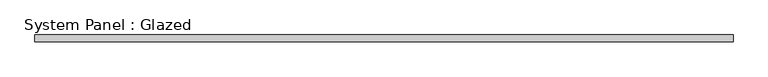
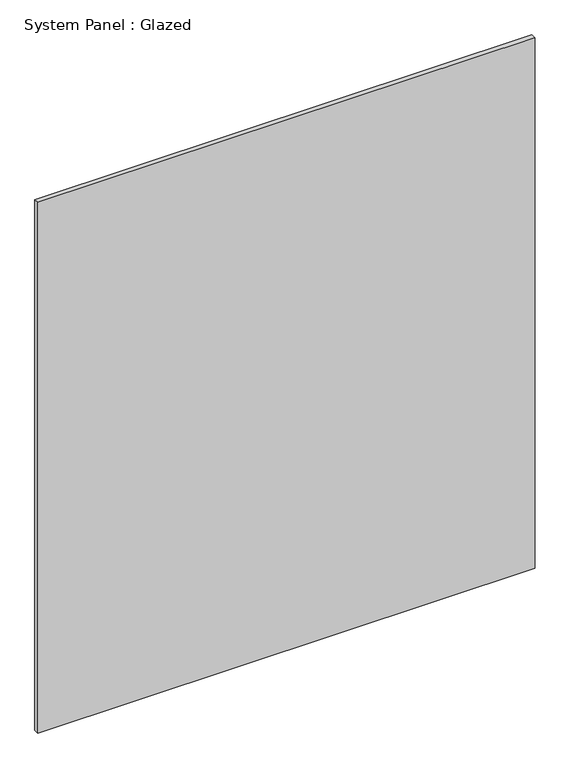
"""IFC4 building model written with IfcOpenShell, lengths in millimetres: plate geometry, System Panel : Glazed."""

from ifc_helpers import new_model, si_unit, origin, origin_with_axes, place, context, project, spatial, polyline, outline, extrude, source, transform, mapped, element, save


def system_panel_glazed_7998c3ce(model_context):
    return source(origin(), model_context, "Body", "SweptSolid", [
        extrude(outline(polyline([(1295.4, 19.05), (-1295.4, 19.05), (-1295.4, 44.45), (1295.4, 44.45), (1295.4, 19.05)])), origin_with_axes(), (0.0, 0.0, 1.0), 2921.0),
    ])


if __name__ == "__main__":
    model = new_model("IFC4")
    model_context = context("Model", 3, world=origin())
    ifc_project = project(units=[si_unit("LENGTHUNIT", "METRE", prefix="MILLI")], contexts=[model_context])
    site = spatial("IfcSite", under=ifc_project)
    building = spatial("IfcBuilding", under=site)
    placement = place(None, origin())
    system_panel_glazed_shape = system_panel_glazed_7998c3ce(model_context)
    element("IfcPlate", 1, ObjectType="System Panel : Glazed", at=placement, inside=building, context=model_context, shape_type="MappedRepresentation", body=[
        mapped(system_panel_glazed_shape, transform((0.0, 0.0, 0.0), x_axis=(1.0, 0.0, 0.0), y_axis=(0.0, 1.0, 0.0), z_axis=(0.0, 0.0, 1.0))),
    ])
    save(model, "model.ifc")

# Revit data of these elements
# Type "System Panel : Glazed"
#   Construction Type Id = "GSP4R"
#   Analytic Construction = "1/8 in Pilkington single glazing"
#   Visual Light Transmittance = 0.9
#   Solar Heat Gain Coefficient = 0.86
#   Heat Transfer Coefficient (U) = 1.18115 BTU/(h·ft²·°F)
#   Define Thermal Properties by = 1
# Element 1 (IfcPlate, "System Panel : Glazed")
#   Materials on its faces: "Glass"
# Materials
#   "Glass": class "Glass", colour RGB 0 128 192, transparency 0.75, Description = "Soda Lime Glass", Cost = 0
